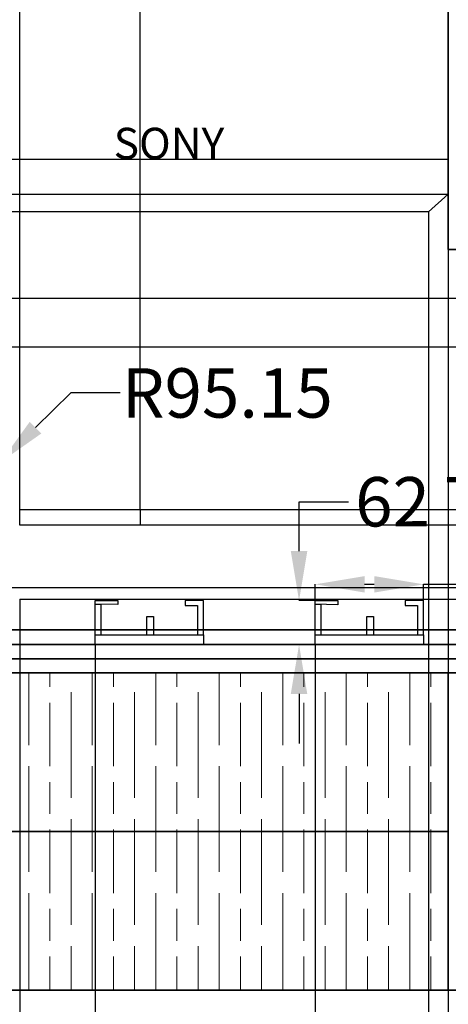
# Model space of a CAD drawing. Units: inches. Extents: x 600 to 5582, y -464 to 3142.
# Tile 5 of 9: x 2777 to 3385, y 532 to 1928. Entities that reach past the tile are written whole.
import ezdxf

# ---------------------------------------------------------------- set-up
doc = ezdxf.new("R2010")
doc.units = ezdxf.units.IN
doc.header["$MEASUREMENT"] = 0
for name, color, linetype, lineweight in [('A-ANNO-DIMS', 2, 'Continuous', 18), ('A-ANNO-TEXT', 7, 'Continuous', 25), ('A-ELEV', 7, 'Continuous', 35), ('A-ELEV-PATT', 252, 'Continuous', 13), ('A-EQPM', 4, 'Continuous', 25)]:
    doc.layers.add(name, color=color, linetype=linetype, lineweight=lineweight)
doc.styles.get("Standard").update_dxf_attribs({"font": 'arial.ttf'})
doc.dimstyles.get("Standard").update_dxf_attribs({"dimtxt": 70, "dimasz": 70, "dimexe": 0.18, "dimexo": 0.0625, "dimgap": 0.09, "dimtad": 0, "dimtih": 1, "dimtoh": 1, "dimdec": 0, "dimzin": 0, "dimdsep": 46, "dimtxsty": 'Standard', "dimcen": 0.09, "dimadec": 0, "dimazin": 0, "dimtfac": 1, "dimtdec": 0, "dimtofl": 0, "dimtmove": 0, "dimatfit": 3, "dimfxl": 1, "dimtolj": 1, "dimtzin": 0, "dimarcsym": 0})

# ---------------------------------------------------------------- blocks, each defined once
blk = doc.blocks.new('HOB-BURNER')
for p, q in [((0, 13.8), (0, 62.4)), ((0, 62.4), (31.8, 62.4)), ((31.8, 56.6), (0, 57.4)), ((0, 57.4), (7.8, 57.2)), ((7.8, 57.2), (7.8, 13.8)), ((31.8, 62.4), (31.8, 56.6)), ((153.5, 62.4), (127.3, 62.4)), ((127.3, 62.4), (127.3, 55.3)), ((153.5, 13.8), (153.5, 62.4)), ((127.3, 55.3), (144.9, 55.3)), ((144.9, 55.3), (144.9, 13.8)), ((73.1, 13.8), (73.1, 39.8)), ((73.1, 39.8), (82.4, 39.8)), ((82.4, 39.8), (82.4, 13.8)), ((7.8, 13.8), (73.1, 13.8)), ((82.4, 13.8), (153.5, 13.8))]:
    blk.add_line(p, q)
blk.add_lwpolyline([(0, 13.8), (153.5, 13.8), (153.5, 0), (0, 0)], close=True)
blk = doc.blocks.new('*D17')
at = {"layer": 'A-ANNO-DIMS', "color": 0, "lineweight": -2, "transparency": 16777216}
for p, q in [((3196.2, 1104.9), (3196.2, 1128.1)), ((3266.2, 1127.9), (3279.8, 1127.9)), ((3349.8, 1104.9), (3349.8, 1128.1)), ((3349.8, 1127.9), (3419.8, 1127.9))]:
    blk.add_line(p, q, dxfattribs=at)
at = {"layer": 'A-ANNO-DIMS', "color": 0, "transparency": 16777216}
for points in [[(3266.2, 1139.5), (3266.2, 1116.2), (3196.2, 1127.9)], [(3279.8, 1139.5), (3279.8, 1116.2), (3349.8, 1127.9)]]:
    blk.add_solid(points, dxfattribs=at)
at = {"layer": 'Defpoints', "color": 0, "transparency": 16777216}
for p in [(3349.8, 1127.9), (3196.2, 1104.9), (3349.8, 1104.9)]:
    blk.add_point(p, dxfattribs=at)
at = {"layer": 'A-ANNO-DIMS', "color": 0, "transparency": 16777216, "insert": (3955.1, 1127.9), "char_height": 70, "attachment_point": 5}
blk.add_mtext('\\A1;HOB BURNER 154 TYP.', dxfattribs=at)
blk = doc.blocks.new('*D18')
at = {"layer": 'A-ANNO-DIMS', "color": 0, "lineweight": -2, "transparency": 16777216}
for p, q in [((3173.2, 1174.9), (3173.2, 1244.9)), ((3173.2, 1244.9), (3243.2, 1244.9)), ((3196.2, 1104.9), (3173, 1104.9)), ((3196.2, 1042.4), (3173, 1042.4)), ((3173.2, 972.4), (3173.2, 902.4))]:
    blk.add_line(p, q, dxfattribs=at)
at = {"layer": 'A-ANNO-DIMS', "color": 0, "transparency": 16777216}
for points in [[(3161.5, 1174.9), (3184.9, 1174.9), (3173.2, 1104.9)], [(3161.5, 972.4), (3184.9, 972.4), (3173.2, 1042.4)]]:
    blk.add_solid(points, dxfattribs=at)
at = {"layer": 'Defpoints', "color": 0, "transparency": 16777216}
for p in [(3173.2, 1104.9), (3196.2, 1104.9), (3196.2, 1042.4)]:
    blk.add_point(p, dxfattribs=at)
at = {"layer": 'A-ANNO-DIMS', "color": 0, "transparency": 16777216, "insert": (3413.9, 1244.9), "char_height": 70, "attachment_point": 5}
blk.add_mtext('\\A1;62 TYP.', dxfattribs=at)
blk = doc.blocks.new('*D25')
at = {"layer": 'A-ANNO-DIMS', "color": 0, "lineweight": -2, "transparency": 16777216}
for p, q in [((2584.7, 1680.8), (2584.7, -233.3)), ((2615, 1655.8), (2615, -233.3)), ((2514.7, -233.1), (2444.7, -233.1)), ((2685, -233.1), (2755, -233.1))]:
    blk.add_line(p, q, dxfattribs=at)
at = {"layer": 'A-ANNO-DIMS', "color": 0, "transparency": 16777216}
for points in [[(2514.7, -221.4), (2514.7, -244.7), (2584.7, -233.1)], [(2685, -221.4), (2685, -244.7), (2615, -233.1)]]:
    blk.add_solid(points, dxfattribs=at)
at = {"layer": 'Defpoints', "color": 0, "transparency": 16777216}
for p in [(2584.7, 1680.8), (2615, 1655.8), (2615, -233.1)]:
    blk.add_point(p, dxfattribs=at)
at = {"layer": 'A-ANNO-DIMS', "color": 0, "transparency": 16777216, "insert": (2873.3, -233.1), "char_height": 70, "attachment_point": 5}
blk.add_mtext('\\A1;30.28', dxfattribs=at)
blk = doc.blocks.new('*D26')
at = {"layer": 'A-ANNO-DIMS', "color": 0, "lineweight": -2, "transparency": 16777216}
for p, q in [((3409.7, 1627.4), (3409.7, -233.3)), ((3384.7, 1602.4), (3384.7, -233.3)), ((3314.7, -233.1), (3244.7, -233.1)), ((3479.7, -233.1), (3549.7, -233.1))]:
    blk.add_line(p, q, dxfattribs=at)
at = {"layer": 'A-ANNO-DIMS', "color": 0, "transparency": 16777216}
for points in [[(3314.7, -221.4), (3314.7, -244.7), (3384.7, -233.1)], [(3479.7, -221.4), (3479.7, -244.7), (3409.7, -233.1)]]:
    blk.add_solid(points, dxfattribs=at)
at = {"layer": 'Defpoints', "color": 0, "transparency": 16777216}
for p in [(3409.7, 1627.4), (3384.7, 1602.4), (3409.7, -233.1)]:
    blk.add_point(p, dxfattribs=at)
at = {"layer": 'A-ANNO-DIMS', "color": 0, "transparency": 16777216, "insert": (3600.8, -233.1), "char_height": 70, "attachment_point": 5}
blk.add_mtext('\\A1;25', dxfattribs=at)
blk = doc.blocks.new('*D57')
at = {"layer": 'A-ANNO-DIMS', "color": 0, "lineweight": -2, "transparency": 16777216}
for p, q in [((5220.2, 622.4), (5220.2, 692.4)), ((5220.2, 692.4), (5290.2, 692.4)), ((1884.8, 552.4), (5220.4, 552.4)), ((1884.8, 512.4), (5220.4, 512.4)), ((5220.2, 442.4), (5220.2, 372.4))]:
    blk.add_line(p, q, dxfattribs=at)
at = {"layer": 'A-ANNO-DIMS', "color": 0, "transparency": 16777216}
for points in [[(5208.6, 622.4), (5231.9, 622.4), (5220.2, 552.4)], [(5208.6, 442.4), (5231.9, 442.4), (5220.2, 512.4)]]:
    blk.add_solid(points, dxfattribs=at)
at = {"layer": 'Defpoints', "color": 0, "transparency": 16777216}
for p in [(1884.7, 552.4), (5220.2, 552.4), (1884.7, 512.4)]:
    blk.add_point(p, dxfattribs=at)
at = {"layer": 'A-ANNO-DIMS', "color": 0, "transparency": 16777216, "insert": (5341.8, 692.4), "char_height": 70, "attachment_point": 5}
blk.add_mtext('\\A1;40', dxfattribs=at)
blk = doc.blocks.new('*D64')
at = {"layer": 'A-ANNO-DIMS', "color": 0, "lineweight": -2, "transparency": 16777216}
for p, q in [((3384.7, 1680.8), (3384.7, -233.3)), ((3356.6, 1655.8), (3356.6, -233.3)), ((3286.6, -233.1), (3216.6, -233.1)), ((3454.7, -233.1), (3524.7, -233.1))]:
    blk.add_line(p, q, dxfattribs=at)
at = {"layer": 'A-ANNO-DIMS', "color": 0, "transparency": 16777216}
for points in [[(3286.6, -221.4), (3286.6, -244.7), (3356.6, -233.1)], [(3454.7, -221.4), (3454.7, -244.7), (3384.7, -233.1)]]:
    blk.add_solid(points, dxfattribs=at)
at = {"layer": 'Defpoints', "color": 0, "transparency": 16777216}
for p in [(3384.7, 1680.8), (3356.6, 1655.8), (3384.7, -233.1)]:
    blk.add_point(p, dxfattribs=at)
at = {"layer": 'A-ANNO-DIMS', "color": 0, "transparency": 16777216, "insert": (3643.5, -233.1), "char_height": 70, "attachment_point": 5}
blk.add_mtext('\\A1;28.17', dxfattribs=at)
blk = doc.blocks.new('*D68')
at = {"layer": 'A-ANNO-DIMS', "color": 0, "lineweight": -2, "transparency": 16777216}
for p, q in [((2777.3, 1106.8), (2777.3, -233.3)), ((2584.7, 1002.4), (2584.7, -233.3)), ((2654.7, -233.1), (2707.3, -233.1)), ((2777.3, -233.1), (2847.3, -233.1))]:
    blk.add_line(p, q, dxfattribs=at)
at = {"layer": 'A-ANNO-DIMS', "color": 0, "transparency": 16777216}
for points in [[(2654.7, -221.4), (2654.7, -244.7), (2584.7, -233.1)], [(2707.3, -221.4), (2707.3, -244.7), (2777.3, -233.1)]]:
    blk.add_solid(points, dxfattribs=at)
at = {"layer": 'Defpoints', "color": 0, "transparency": 16777216}
for p in [(2777.3, 1106.8), (2584.7, 1002.4), (2777.3, -233.1)]:
    blk.add_point(p, dxfattribs=at)
at = {"layer": 'A-ANNO-DIMS', "color": 0, "transparency": 16777216, "insert": (2982.6, -233.1), "char_height": 70, "attachment_point": 5}
blk.add_mtext('\\A1;192.51', dxfattribs=at)
blk = doc.blocks.new('*D69')
at = {"layer": 'A-ANNO-DIMS', "color": 0, "lineweight": -2, "transparency": 16777216}
for p, q in [((5220.2, 1304), (5220.2, 1374)), ((2777.3, 1234), (5220.4, 1234)), ((2777.3, 1106.8), (5220.4, 1106.8)), ((5220.2, 1036.8), (5220.2, 966.8))]:
    blk.add_line(p, q, dxfattribs=at)
at = {"layer": 'A-ANNO-DIMS', "color": 0, "transparency": 16777216}
for points in [[(5208.6, 1304), (5231.9, 1304), (5220.2, 1234)], [(5208.6, 1036.8), (5231.9, 1036.8), (5220.2, 1106.8)]]:
    blk.add_solid(points, dxfattribs=at)
at = {"layer": 'Defpoints', "color": 0, "transparency": 16777216}
for p in [(2777.3, 1234), (5220.2, 1234), (2777.3, 1106.8)]:
    blk.add_point(p, dxfattribs=at)
at = {"layer": 'A-ANNO-DIMS', "color": 0, "transparency": 16777216, "insert": (5220.2, 1170.4), "char_height": 70, "attachment_point": 5}
blk.add_mtext('\\A1;127.21', dxfattribs=at)
blk = doc.blocks.new('*D71')
at = {"layer": 'A-ANNO-DIMS', "color": 0, "lineweight": -2, "transparency": 16777216}
for p, q in [((2777.3, 1234.1), (2777.3, 2988.1)), ((2847.3, 2987.9), (2877.8, 2987.9)), ((2947.8, 1234.1), (2947.8, 2988.1)), ((2947.8, 2987.9), (3017.8, 2987.9))]:
    blk.add_line(p, q, dxfattribs=at)
at = {"layer": 'A-ANNO-DIMS', "color": 0, "transparency": 16777216}
for points in [[(2847.3, 2999.6), (2847.3, 2976.3), (2777.3, 2987.9)], [(2877.8, 2999.6), (2877.8, 2976.3), (2947.8, 2987.9)]]:
    blk.add_solid(points, dxfattribs=at)
at = {"layer": 'Defpoints', "color": 0, "transparency": 16777216}
for p in [(2947.8, 2987.9), (2777.3, 1234), (2947.8, 1234)]:
    blk.add_point(p, dxfattribs=at)
at = {"layer": 'A-ANNO-DIMS', "color": 0, "transparency": 16777216, "insert": (3160, 2987.9), "char_height": 70, "attachment_point": 5}
blk.add_mtext('\\A1;170.59', dxfattribs=at)
blk = doc.blocks.new('*D72')
at = {"layer": 'A-ANNO-DIMS', "color": 0, "lineweight": -2, "transparency": 16777216}
for p, q in [((5220.2, 1304), (5220.2, 1374)), ((5220.2, 1374), (5290.2, 1374)), ((2947.9, 1234), (5220.4, 1234)), ((2947.9, 1212), (5220.4, 1212)), ((5220.2, 1142), (5220.2, 1072))]:
    blk.add_line(p, q, dxfattribs=at)
at = {"layer": 'A-ANNO-DIMS', "color": 0, "transparency": 16777216}
for points in [[(5208.6, 1304), (5231.9, 1304), (5220.2, 1234)], [(5208.6, 1142), (5231.9, 1142), (5220.2, 1212)]]:
    blk.add_solid(points, dxfattribs=at)
at = {"layer": 'Defpoints', "color": 0, "transparency": 16777216}
for p in [(2947.8, 1234), (5220.2, 1234), (2947.8, 1212)]:
    blk.add_point(p, dxfattribs=at)
at = {"layer": 'A-ANNO-DIMS', "color": 0, "transparency": 16777216, "insert": (5436.2, 1374), "char_height": 70, "attachment_point": 5}
blk.add_mtext('\\A1;22.087', dxfattribs=at)
blk = doc.blocks.new('*D73')
at = {"layer": 'A-ANNO-DIMS', "color": 0, "lineweight": -2, "transparency": 16777216}
for p, q in [((2599.2, 1042.4), (2599.2, -233.3)), ((2584.7, 1002.4), (2584.7, -233.3)), ((2514.7, -233.1), (2444.7, -233.1)), ((2669.2, -233.1), (2739.2, -233.1))]:
    blk.add_line(p, q, dxfattribs=at)
at = {"layer": 'A-ANNO-DIMS', "color": 0, "transparency": 16777216}
for points in [[(2514.7, -221.4), (2514.7, -244.7), (2584.7, -233.1)], [(2669.2, -221.4), (2669.2, -244.7), (2599.2, -233.1)]]:
    blk.add_solid(points, dxfattribs=at)
at = {"layer": 'Defpoints', "color": 0, "transparency": 16777216}
for p in [(2599.2, 1042.4), (2584.7, 1002.4), (2599.2, -233.1)]:
    blk.add_point(p, dxfattribs=at)
at = {"layer": 'A-ANNO-DIMS', "color": 0, "transparency": 16777216, "insert": (2854, -233.1), "char_height": 70, "attachment_point": 5}
blk.add_mtext('\\A1;14.50', dxfattribs=at)
blk = doc.blocks.new('*D74')
at = {"layer": 'A-ANNO-DIMS', "color": 0, "lineweight": -2, "transparency": 16777216}
for p, q in [((2599.2, 1042.4), (2599.2, -233.3)), ((2884.4, 1042.4), (2884.4, -233.3)), ((2669.2, -233.1), (2814.4, -233.1)), ((2884.4, -233.1), (2954.4, -233.1))]:
    blk.add_line(p, q, dxfattribs=at)
at = {"layer": 'A-ANNO-DIMS', "color": 0, "transparency": 16777216}
for points in [[(2669.2, -221.4), (2669.2, -244.7), (2599.2, -233.1)], [(2814.4, -221.4), (2814.4, -244.7), (2884.4, -233.1)]]:
    blk.add_solid(points, dxfattribs=at)
at = {"layer": 'Defpoints', "color": 0, "transparency": 16777216}
for p in [(2599.2, 1042.4), (2884.4, 1042.4), (2884.4, -233.1)]:
    blk.add_point(p, dxfattribs=at)
at = {"layer": 'A-ANNO-DIMS', "color": 0, "transparency": 16777216, "insert": (3100, -233.1), "char_height": 70, "attachment_point": 5}
blk.add_mtext('\\A1;285.12', dxfattribs=at)
blk = doc.blocks.new('*D75')
at = {"layer": 'A-ANNO-DIMS', "color": 0, "lineweight": -2, "transparency": 16777216}
for p, q in [((2884.4, 1042.4), (2884.4, -233.3)), ((3196.2, 1042.4), (3196.2, -233.3)), ((2814.4, -233.1), (2744.4, -233.1)), ((3266.2, -233.1), (3336.2, -233.1))]:
    blk.add_line(p, q, dxfattribs=at)
at = {"layer": 'A-ANNO-DIMS', "color": 0, "transparency": 16777216}
for points in [[(2814.4, -221.4), (2814.4, -244.7), (2884.4, -233.1)], [(3266.2, -221.4), (3266.2, -244.7), (3196.2, -233.1)]]:
    blk.add_solid(points, dxfattribs=at)
at = {"layer": 'Defpoints', "color": 0, "transparency": 16777216}
for p in [(2884.4, 1042.4), (3196.2, 1042.4), (3196.2, -233.1)]:
    blk.add_point(p, dxfattribs=at)
at = {"layer": 'A-ANNO-DIMS', "color": 0, "transparency": 16777216, "insert": (3040.3, -233.1), "char_height": 70, "attachment_point": 5}
blk.add_mtext('\\A1;311.87', dxfattribs=at)
blk = doc.blocks.new('*D81')
at = {"layer": 'A-ANNO-DIMS', "color": 0, "lineweight": -2, "transparency": 16777216}
for p, q in [((5220.2, 1133.7), (5220.2, 1203.7)), ((5220.2, 1203.7), (5290.2, 1203.7)), ((2292.1, 1063.7), (5220.4, 1063.7)), ((2310.1, 1042.4), (5220.4, 1042.4)), ((5220.2, 972.4), (5220.2, 902.4))]:
    blk.add_line(p, q, dxfattribs=at)
at = {"layer": 'A-ANNO-DIMS', "color": 0, "transparency": 16777216}
for points in [[(5208.6, 1133.7), (5231.9, 1133.7), (5220.2, 1063.7)], [(5208.6, 972.4), (5231.9, 972.4), (5220.2, 1042.4)]]:
    blk.add_solid(points, dxfattribs=at)
at = {"layer": 'Defpoints', "color": 0, "transparency": 16777216}
for p in [(2292, 1063.7), (5220.2, 1063.7), (2310, 1042.4)]:
    blk.add_point(p, dxfattribs=at)
at = {"layer": 'A-ANNO-DIMS', "color": 0, "transparency": 16777216, "insert": (5409, 1203.7), "char_height": 70, "attachment_point": 5}
blk.add_mtext('\\A1;21.26', dxfattribs=at)
blk = doc.blocks.new('*D85')
at = {"layer": 'A-ANNO-DIMS', "color": 0, "lineweight": -2, "transparency": 16777216}
for p, q in [((5220.2, 1193.3), (5220.2, 1263.3)), ((5220.2, 1263.3), (5290.2, 1263.3)), ((2231.9, 1123.3), (5220.4, 1123.3)), ((2232.3, 1063.4), (5220.4, 1063.4)), ((5220.2, 993.4), (5220.2, 923.4))]:
    blk.add_line(p, q, dxfattribs=at)
at = {"layer": 'A-ANNO-DIMS', "color": 0, "transparency": 16777216}
for points in [[(5208.6, 1193.3), (5231.9, 1193.3), (5220.2, 1123.3)], [(5208.6, 993.4), (5231.9, 993.4), (5220.2, 1063.4)]]:
    blk.add_solid(points, dxfattribs=at)
at = {"layer": 'Defpoints', "color": 0, "transparency": 16777216}
for p in [(2231.8, 1123.3), (5220.2, 1123.3), (2232.2, 1063.4)]:
    blk.add_point(p, dxfattribs=at)
at = {"layer": 'A-ANNO-DIMS', "color": 0, "transparency": 16777216, "insert": (5408.5, 1263.3), "char_height": 70, "attachment_point": 5}
blk.add_mtext('\\A1;59.99', dxfattribs=at)
blk = doc.blocks.new('*D94')
at = {"layer": 'A-ANNO-DIMS', "color": 0, "lineweight": -2, "transparency": 16777216}
for p, q in [((2340.4, 1533.4), (2340.4, -233.3)), ((2411.7, 1533.4), (2411.7, -233.3)), ((2270.4, -233.1), (2200.4, -233.1)), ((2481.7, -233.1), (2551.7, -233.1))]:
    blk.add_line(p, q, dxfattribs=at)
at = {"layer": 'A-ANNO-DIMS', "color": 0, "transparency": 16777216}
for points in [[(2270.4, -221.4), (2270.4, -244.7), (2340.4, -233.1)], [(2481.7, -221.4), (2481.7, -244.7), (2411.7, -233.1)]]:
    blk.add_solid(points, dxfattribs=at)
at = {"layer": 'Defpoints', "color": 0, "transparency": 16777216}
for p in [(2340.4, 1533.5), (2411.7, 1533.5), (2411.7, -233.1)]:
    blk.add_point(p, dxfattribs=at)
at = {"layer": 'A-ANNO-DIMS', "color": 0, "transparency": 16777216, "insert": (2669.5, -233.1), "char_height": 70, "attachment_point": 5}
blk.add_mtext('\\A1;71.34', dxfattribs=at)
blk = doc.blocks.new('*D95')
at = {"layer": 'A-ANNO-DIMS', "color": 0, "lineweight": -2, "transparency": 16777216}
for p, q in [((2411.7, 1533.4), (2411.7, -233.3)), ((2465.8, 1533.4), (2465.8, -233.3)), ((2341.7, -233.1), (2271.7, -233.1)), ((2535.8, -233.1), (2605.8, -233.1))]:
    blk.add_line(p, q, dxfattribs=at)
at = {"layer": 'A-ANNO-DIMS', "color": 0, "transparency": 16777216}
for points in [[(2341.7, -221.4), (2341.7, -244.7), (2411.7, -233.1)], [(2535.8, -221.4), (2535.8, -244.7), (2465.8, -233.1)]]:
    blk.add_solid(points, dxfattribs=at)
at = {"layer": 'Defpoints', "color": 0, "transparency": 16777216}
for p in [(2411.7, 1533.5), (2465.8, 1533.5), (2465.8, -233.1)]:
    blk.add_point(p, dxfattribs=at)
at = {"layer": 'A-ANNO-DIMS', "color": 0, "transparency": 16777216, "insert": (2724, -233.1), "char_height": 70, "attachment_point": 5}
blk.add_mtext('\\A1;54.13', dxfattribs=at)
blk = doc.blocks.new('*D96')
at = {"layer": 'A-ANNO-DIMS', "color": 0, "lineweight": -2, "transparency": 16777216}
for p, q in [((2465.8, 1533.4), (2465.8, -233.3)), ((2539.2, 1533.4), (2539.2, -233.3)), ((2395.8, -233.1), (2325.8, -233.1)), ((2609.2, -233.1), (2679.2, -233.1))]:
    blk.add_line(p, q, dxfattribs=at)
at = {"layer": 'A-ANNO-DIMS', "color": 0, "transparency": 16777216}
for points in [[(2395.8, -221.4), (2395.8, -244.7), (2465.8, -233.1)], [(2609.2, -221.4), (2609.2, -244.7), (2539.2, -233.1)]]:
    blk.add_solid(points, dxfattribs=at)
at = {"layer": 'Defpoints', "color": 0, "transparency": 16777216}
for p in [(2465.8, 1533.5), (2539.2, 1533.5), (2539.2, -233.1)]:
    blk.add_point(p, dxfattribs=at)
at = {"layer": 'A-ANNO-DIMS', "color": 0, "transparency": 16777216, "insert": (2797.1, -233.1), "char_height": 70, "attachment_point": 5}
blk.add_mtext('\\A1;73.33', dxfattribs=at)
blk = doc.blocks.new('*D99')
at = {"layer": 'A-ANNO-DIMS', "color": 0, "lineweight": -2, "transparency": 16777216}
for p, q in [((5220.2, 1603.5), (5220.2, 1673.5)), ((2271, 1533.5), (5220.4, 1533.5)), ((2273, 1464.8), (5220.4, 1464.8)), ((5220.2, 1394.8), (5220.2, 1324.8)), ((5220.2, 1324.8), (5150.2, 1324.8))]:
    blk.add_line(p, q, dxfattribs=at)
at = {"layer": 'A-ANNO-DIMS', "color": 0, "transparency": 16777216}
for points in [[(5208.6, 1603.5), (5231.9, 1603.5), (5220.2, 1533.5)], [(5208.6, 1394.8), (5231.9, 1394.8), (5220.2, 1464.8)]]:
    blk.add_solid(points, dxfattribs=at)
at = {"layer": 'Defpoints', "color": 0, "transparency": 16777216}
for p in [(2271, 1533.5), (2272.9, 1464.8), (5220.2, 1464.8)]:
    blk.add_point(p, dxfattribs=at)
at = {"layer": 'A-ANNO-DIMS', "color": 0, "transparency": 16777216, "insert": (5038.6, 1324.8), "char_height": 70, "attachment_point": 5}
blk.add_mtext('\\A1;68.71', dxfattribs=at)
blk = doc.blocks.new('*D103')
at = {"layer": 'A-ANNO-DIMS', "color": 0, "lineweight": -2, "transparency": 16777216}
for p, q in [((2849.5, 1399.2), (2799.7, 1350)), ((2919.5, 1399.2), (2849.5, 1399.2)), ((2682, 1234), (2682.2, 1234)), ((2682.1, 1234), (2682.1, 1234.1))]:
    blk.add_line(p, q, dxfattribs=at)
at = {"layer": 'A-ANNO-DIMS', "color": 0, "transparency": 16777216}
blk.add_solid([(2791.5, 1358.3), (2807.9, 1341.7), (2749.9, 1300.9)], dxfattribs=at)
at = {"layer": 'Defpoints', "color": 0, "transparency": 16777216}
for p in [(2749.9, 1300.9), (2682.1, 1234)]:
    blk.add_point(p, dxfattribs=at)
at = {"layer": 'A-ANNO-DIMS', "color": 0, "transparency": 16777216, "insert": (3071.5, 1399.2), "char_height": 70, "attachment_point": 5}
blk.add_mtext('\\A1;R95.15', dxfattribs=at)

msp = doc.modelspace()

# ---------------------------------------------------------------- hatches: boundary and pattern name
at = {"layer": 'A-ELEV-PATT'}
h = msp.add_hatch(dxfattribs=at)
h.set_pattern_fill('GOST_WOOD', color=256, scale=15)
h.set_pattern_definition([(90, (0, 0), (90, -6e-15), [150, -30]), (90, (30, -30), (90, -6e-15), [90, -22.5, 45, -22.5]), (90, (60, -75), (90, -6e-15), [150, -30])])
h.paths.add_polyline_path([(4959.7485, 2752.4212), (1409.7485, 2752.4212), (1409.7485, 2352.4212), (1784.7485, 2352.4212), (4959.7485, 2352.4212)])
h.paths.add_polyline_path([(3384.7485, 1002.4212), (2584.7485, 1002.4212), (2584.7485, 777.4212), (3384.7485, 777.4212)])
h.paths.add_polyline_path([(3384.7485, 777.4212), (2584.7485, 777.4212), (2584.7485, 552.4212), (3384.7485, 552.4212)])
h.paths.add_polyline_path([(3384.7485, 512.4212), (2584.7485, 512.4212), (2584.7485, 102.4212), (3384.7485, 102.4212)])
h = msp.add_hatch(dxfattribs=at)
h.set_pattern_fill('CROSS', color=256, scale=100)
h.paths.add_polyline_path([(1759.7485, 2327.4212), (1409.7485, 2327.4212), (1409.7485, 1967.4212), (1759.7485, 1967.4212)])
h.paths.add_polyline_path([(1759.7485, 1952.4212), (1409.7485, 1952.4212), (1409.7485, 1567.4212), (1759.7485, 1567.4212)])
h.paths.add_polyline_path([(1759.7485, 1552.4212), (1409.7485, 1552.4212), (1409.7485, 1167.4212), (1759.7485, 1167.4212)])
h.paths.add_polyline_path([(1759.7485, 1152.4212), (1409.7485, 1152.4212), (1409.7485, 767.4212), (1759.7485, 767.4212)])
h.paths.add_polyline_path([(1759.7485, 752.4212), (1409.7485, 752.4212), (1409.7485, 367.4212), (1759.7485, 367.4212)])
h.paths.add_polyline_path([(1759.7485, 352.4212), (1409.7485, 352.4212), (1409.7485, 142.4212), (1759.7485, 142.4212)])
h.paths.add_polyline_path([(3759.7485, 1977.4212), (3409.7485, 1977.4212), (3409.7485, 1627.4212), (3759.7485, 1627.4212)])
h.paths.add_polyline_path([(3714.7508, 1954.858, -1), (3750.8891, 1954.858, -1)], flags=16)
h.paths.add_polyline_path([(3759.7485, 2327.4212), (3409.7485, 2327.4212), (3409.7485, 2002.4212), (3759.7485, 2002.4212)])
h.paths.add_polyline_path([(4159.7485, 2327.4212), (3809.7485, 2327.4212), (3809.7485, 2002.4212), (4159.7485, 2002.4212)])
h.paths.add_polyline_path([(4159.7485, 1977.4212), (3809.7485, 1977.4212), (3813.5467, 1954.858, -1), (3849.685, 1954.858, -1), (3813.5467, 1954.858), (3809.7485, 1627.4212), (4159.7485, 1627.4212)])
h.paths.add_polyline_path([(4559.7485, 2327.4212), (4184.7485, 2327.4212), (4184.7485, 2002.4212), (4559.7485, 2002.4212)])
h.paths.add_polyline_path([(4559.7485, 1977.4212), (4184.7485, 1977.4212), (4184.7485, 1627.4212), (4559.7485, 1627.4212)])
h.paths.add_polyline_path([(4517.0704, 1954.858, -1), (4553.2087, 1954.858, -1)], flags=16)
h.paths.add_polyline_path([(4959.7485, 2327.4212), (4609.7485, 2327.4212), (4609.7485, 2002.4212), (4959.7485, 2002.4212)])
h.paths.add_polyline_path([(4959.7485, 1977.4212), (4609.7485, 1977.4212), (4609.7485, 1627.4212), (4959.7485, 1627.4212)])
h.paths.add_polyline_path([(4619.5464, 1954.858, -1), (4655.6847, 1954.858, -1)], flags=16)

# ---------------------------------------------------------------- linework, layer by layer
at = {"layer": 'A-ELEV'}
for p, q in [((4984.7485, 1042.4212), (1784.7485, 1042.4212)), ((4984.7485, 1022.4212), (1784.7485, 1022.4212)), ((4984.7485, 1002.4212), (1784.7485, 1002.4212)), ((3384.7485, 552.4212), (3384.7485, 1002.4212)), ((2584.7485, 777.4212), (3384.7485, 777.4212)), ((4184.7485, 552.4212), (1884.7485, 552.4212))]:
    msp.add_line(p, q, dxfattribs=at)
msp.add_lwpolyline([(4984.7485, 1602.4212), (3384.7485, 1602.4212), (3384.7485, 2352.4212), (3784.7485, 2352.4212)], dxfattribs=at)
at = {"layer": 'A-EQPM'}
for p, q in [((2584.7485, 1730.8271), (3384.7485, 1730.8271)), ((2884.371, 1056.1771), (2884.371, 1104.8519)), ((2884.371, 1104.8519), (2916.135, 1104.8519)), ((2916.135, 1104.8519), (2916.135, 1099.0604)), ((2916.135, 1099.0604), (2884.371, 1099.8376)), ((2884.371, 1099.8376), (2892.1537, 1099.6472)), ((2892.1537, 1099.6472), (2892.1537, 1056.1771))]:
    msp.add_line(p, q, dxfattribs=at)
for points in [[(3384.7485, 1680.8271), (3356.5781, 1655.8271), (2615.026, 1655.8271), (2584.7485, 1680.8271)], [(2777.2556, 1234.0488), (2947.8448, 1234.0488), (2947.8448, 1211.9616), (2777.2556, 1211.9616)], [(2884.371, 1056.1771), (3037.8972, 1056.1771), (3037.8972, 1042.4212), (2884.371, 1042.4212)]]:
    msp.add_lwpolyline(points, close=True, dxfattribs=at)
for points in [[(3037.8972, 1056.1771), (3037.8972, 1104.8519), (3011.6249, 1104.8519), (3011.6249, 1097.765), (3029.2525, 1097.765), (3029.2525, 1056.1771)], [(2957.446, 1056.1771), (2957.446, 1082.2209), (2966.7783, 1082.2209), (2966.7783, 1056.1771)]]:
    msp.add_lwpolyline(points, dxfattribs=at)

# ---------------------------------------------------------------- block references
msp.add_blockref('HOB-BURNER', (3196.2384, 1042.4211), dxfattribs=at)

# ---------------------------------------------------------------- texts
at = {"layer": 'A-ANNO-TEXT'}
msp.add_text('SONY ', height=44.32617, dxfattribs=at).set_placement((2910.3971, 1730.8271))

# ---------------------------------------------------------------- dimensions: what is measured, and where the dimension line sits
at = {"layer": 'A-ANNO-DIMS'}
for base, p1, p2, override, picture, middle in [((2947.8448, 2987.9212), (2777.2556, 1234.0488), (2947.8448, 1234.0488), {"dimdec": 2, "dimlfac": 1, "dimrnd": 0, "dimzin": 0, "dimdsep": 46, "dimlunit": 2}, '*D71', (3160.0119, 2987.9212)), ((2615.026, -233.0788), (2584.7485, 1680.8271), (2615.026, 1655.8271), {"dimdec": 2, "dimlfac": 1, "dimrnd": 0, "dimzin": 0, "dimdsep": 46, "dimlunit": 2}, '*D25', (2873.2709, -233.0788)), ((3384.7485, -233.0788), (3356.5781, 1655.8271), (3384.7485, 1680.8271), {"dimdec": 2, "dimlfac": 1, "dimrnd": 0, "dimzin": 0, "dimdsep": 46, "dimlunit": 2}, '*D64', (3643.5424, -233.0788)), ((3409.7485, -233.0788), (3384.7485, 1602.4212), (3409.7485, 1627.4212), {"dimdec": 0, "dimlfac": 1, "dimrnd": 0, "dimzin": 0, "dimdsep": 46, "dimlunit": 2}, '*D26', (3600.8344, -233.0788)), ((2411.7034, -233.0788), (2340.3598, 1533.4874), (2411.7034, 1533.4874), {"dimdec": 2, "dimlfac": 1, "dimrnd": 0, "dimzin": 0, "dimdsep": 46, "dimlunit": 2}, '*D94', (2669.4707, -233.0788)), ((2465.8357, -233.0788), (2411.7034, 1533.4874), (2465.8357, 1533.4874), {"dimdec": 2, "dimlfac": 1, "dimrnd": 0, "dimzin": 0, "dimdsep": 46, "dimlunit": 2}, '*D95', (2724.0328, -233.0788)), ((2539.1643, -233.0788), (2465.8357, 1533.4874), (2539.1643, 1533.4874), {"dimdec": 2, "dimlfac": 1, "dimrnd": 0, "dimzin": 0, "dimdsep": 46, "dimlunit": 2}, '*D96', (2797.0749, -233.0788)), ((2777.2556, -233.0788), (2584.7485, 1002.4212), (2777.2556, 1106.8415), {"dimdec": 2, "dimlfac": 1, "dimrnd": 0, "dimzin": 0, "dimdsep": 46, "dimlunit": 2}, '*D68', (2982.5946, -233.0788)), ((2599.2497, -233.0788), (2584.7485, 1002.4212), (2599.2497, 1042.42), {"dimdec": 2, "dimlfac": 1, "dimrnd": 0, "dimzin": 0, "dimdsep": 46, "dimlunit": 2}, '*D73', (2854.0327, -233.0788)), ((2884.371, -233.0788), (2599.2497, 1042.42), (2884.371, 1042.4212), {"dimdec": 2, "dimlfac": 1, "dimrnd": 0, "dimzin": 0, "dimdsep": 46, "dimlunit": 2}, '*D74', (3099.9999, -233.0788)), ((3196.2381, -233.0788), (2884.371, 1042.4212), (3196.2381, 1042.4212), {"dimdec": 2, "dimlfac": 1, "dimrnd": 0, "dimzin": 0, "dimdsep": 46, "dimlunit": 2}, '*D75', (3040.3046, -233.0788))]:
    dim = msp.add_linear_dim(base=base, p1=p1, p2=p2, dimstyle='Standard', override=override, dxfattribs=at)
    dim.commit()
    dim.dimension.update_dxf_attribs({"geometry": picture, "text_midpoint": middle})
for base, p1, p2, override, picture, middle in [((5220.2485, 1464.7817), (2270.9593, 1533.4874), (2272.9025, 1464.7817), {"dimdec": 2, "dimlfac": 1, "dimrnd": 0, "dimzin": 0, "dimdsep": 46, "dimlunit": 2}, '*D99', (5038.6169, 1324.7817)), ((5220.2485, 1234.0488), (2947.8448, 1211.9616), (2947.8448, 1234.0488), {"dimdec": 3, "dimlfac": 1, "dimrnd": 0, "dimzin": 0, "dimdsep": 46, "dimlunit": 2}, '*D72', (5436.2355, 1374.0488)), ((5220.2485, 1234.0488), (2777.2556, 1106.8415), (2777.2556, 1234.0488), {"dimdec": 2, "dimlfac": 1, "dimrnd": 0, "dimzin": 0, "dimdsep": 46, "dimlunit": 2}, '*D69', (5220.2485, 1170.4451)), ((5220.2485, 1123.3472), (2232.228, 1063.362), (2231.8275, 1123.3472), {"dimdec": 2, "dimlfac": 1, "dimrnd": 0, "dimzin": 0, "dimdsep": 46, "dimlunit": 2}, '*D85', (5408.5172, 1263.3472)), ((5220.2485, 1063.682), (2310.0444, 1042.4212), (2292.0448, 1063.682), {"dimdec": 2, "dimlfac": 1, "dimrnd": 0, "dimzin": 0, "dimdsep": 46, "dimlunit": 2}, '*D81', (5409.0186, 1203.682)), ((5220.2485, 552.4212), (1884.7485, 512.4212), (1884.7485, 552.4212), {"dimdec": 0, "dimlfac": 1, "dimrnd": 0, "dimzin": 0, "dimdsep": 46, "dimlunit": 2}, '*D57', (5341.7641, 692.4212))]:
    dim = msp.add_linear_dim(base=base, p1=p1, p2=p2, angle=90, dimstyle='Standard', override=override, dxfattribs=at)
    dim.commit()
    dim.dimension.update_dxf_attribs({"geometry": picture, "text_midpoint": middle})
dim = msp.add_radius_dim(center=(2682.10062, 1234.04876), mpoint=(2749.85675, 1300.85875), dimstyle='Standard', override={"dimdec": 2, "dimlfac": 1, "dimrnd": 0, "dimzin": 0, "dimdsep": 46, "dimlunit": 2}, dxfattribs=at)
dim.commit()
dim.dimension.update_dxf_attribs({"geometry": '*D103', "text_midpoint": (3071.5009, 1399.15523)})
dim = msp.add_linear_dim(base=(3173.2092, 1104.8519), p1=(3196.2381, 1042.4212), p2=(3196.2381, 1104.8519), angle=90, text='<> TYP.', dimstyle='Standard', override={"dimdec": 0, "dimrnd": 0, "dimzin": 0, "dimlunit": 2}, dxfattribs=at)
dim.commit()
dim.dimension.update_dxf_attribs({"geometry": '*D18', "text_midpoint": (3413.8585, 1244.8519)})
dim = msp.add_linear_dim(base=(3349.7642, 1127.8808), p1=(3196.2381, 1104.8519), p2=(3349.7642, 1104.8519), text='HOB BURNER <> TYP.', dimstyle='Standard', override={"dimdec": 0, "dimrnd": 0, "dimzin": 0, "dimlunit": 2}, dxfattribs=at)
dim.commit()
dim.dimension.update_dxf_attribs({"geometry": '*D17', "text_midpoint": (3955.1203, 1127.8808)})

doc.saveas('drawing.dxf')
